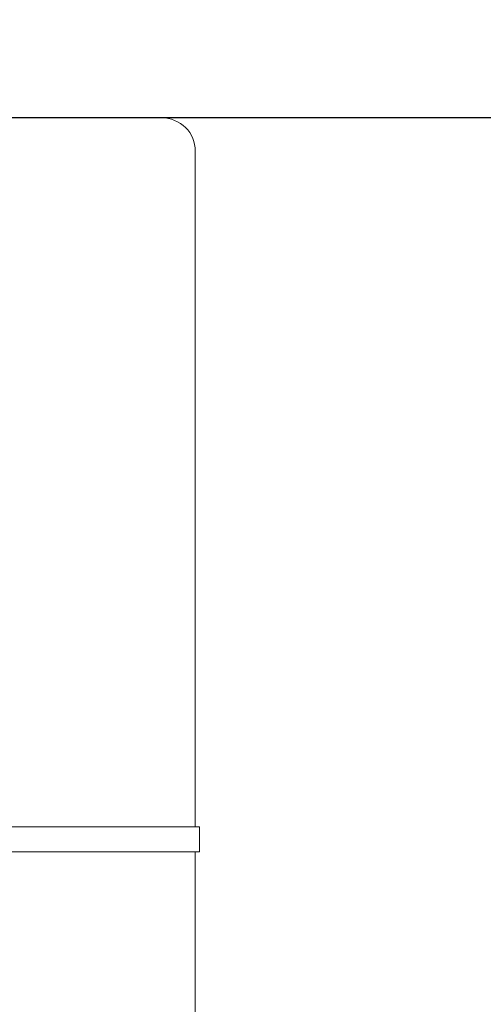
# Model space of a CAD drawing. Units: inches. Extents: x -1198 to -69, y -512 to 437.
# Tile 37 of 50: x -625.117 to -622.655, y 180.515 to 185.749. Entities that reach past the tile are written whole.
import ezdxf

# ---------------------------------------------------------------- set-up
doc = ezdxf.new("R2010")
doc.units = ezdxf.units.IN
doc.header["$MEASUREMENT"] = 0
for name, color, linetype, lineweight in [('0_Pen_No__7', 7, 'Continuous', 18), ('A-ANNO-DIMS', 2, 'Continuous', 18), ('A-EQPM', 60, 'Continuous', 18), ('A-FLOR-CASE', 7, 'Continuous', 25)]:
    doc.layers.add(name, color=color, linetype=linetype, lineweight=lineweight)
doc.styles.get("Standard").update_dxf_attribs({"font": 'arial.ttf'})
doc.dimstyles.get("Standard").update_dxf_attribs({"dimtxt": 6, "dimasz": 6, "dimexe": 0.18, "dimexo": 0.0625, "dimgap": 0.09, "dimtad": 0, "dimtih": 1, "dimtoh": 1, "dimdec": 0, "dimzin": 0, "dimdsep": 46, "dimlunit": 4, "dimtxsty": 'Standard', "dimblk": 'OBLIQUE', "dimcen": 0.09, "dimadec": 0, "dimazin": 0, "dimtfac": 1, "dimtdec": 0, "dimtofl": 0, "dimtmove": 0, "dimatfit": 3, "dimfxl": 1, "dimtolj": 1, "dimtzin": 0, "dimarcsym": 0})

# ---------------------------------------------------------------- blocks, each defined once
blk = doc.blocks.new('new block')
at = {"layer": '0_Pen_No__7'}
for p, q in [((-359, 99.11), (485.68, 99.11)), ((485.68, 95.73), (-359, 95.73))]:
    blk.add_line(p, q, dxfattribs=at)
blk.add_lwpolyline([(-354.49, 596.91), (481.18, 596.91, -0.414214), (485.68, 592.4), (485.68, 99.11), (486.24, 99.11), (486.24, 95.73), (485.68, 95.73), (485.68, 4.5, -0.414214), (481.18, 0), (-354.49, 0, -0.414214), (-359, 4.5), (-359, 95.73), (-359.56, 95.73), (-359.56, 99.11), (-359, 99.11), (-359, 592.4, -0.414214)], format="xyb", close=True, dxfattribs=at)
blk = doc.blocks.new('COUNTER-L')
at = {"ltscale": 10}
blk.add_line((49.3491, 23.9997), (0.0001, 23.9997), dxfattribs=at)
blk = doc.blocks.new('_Oblique')
at = {"color": 0, "linetype": 'ByBlock', "lineweight": -2}
blk.add_line((-0.5, -0.5), (0.5, 0.5), dxfattribs=at)
blk = doc.blocks.new('*D56')
at = {"layer": 'A-ANNO-DIMS', "color": 0, "lineweight": -2, "ltscale": 10, "transparency": 16777216}
for p, q in [((-618.3394, 257.2277), (-603.8219, 257.2277)), ((-604.0019, 257.2277), (-604.0019, 212.422)), ((-604.0019, 161.2277), (-604.0019, 206.0333)), ((-618.3394, 161.2277), (-603.8219, 161.2277))]:
    blk.add_line(p, q, dxfattribs=at)
at = {"layer": 'DEFPOINTS', "color": 0, "ltscale": 10, "transparency": 16777216}
for p in [(-618.4019, 257.2277), (-604.0019, 257.2277), (-618.4019, 161.2277)]:
    blk.add_point(p, dxfattribs=at)
at = {"layer": 'A-ANNO-DIMS', "color": 0, "lineweight": -2, "ltscale": 10, "transparency": 16777216, "xscale": 6, "yscale": 6, "zscale": 6}
for p, rotation in [((-604.0019, 257.2277), 90), ((-604.0019, 161.2277), 270)]:
    blk.add_blockref('_Oblique', p, dxfattribs=dict(at, rotation=rotation))
at = {"layer": 'A-ANNO-DIMS', "color": 0, "ltscale": 10, "transparency": 16777216, "insert": (-604.0019, 209.2277), "char_height": 6, "attachment_point": 5}
blk.add_mtext('\\A1;COUNTER 96 TYP.', dxfattribs=at)

msp = doc.modelspace()

# ---------------------------------------------------------------- block references
at = {"layer": 'A-EQPM', "xscale": 0.0393700787401575, "yscale": 0.0393700787401575, "zscale": 0.0393700787401575, "rotation": 180}
msp.add_blockref('new block', (-638.3186, 185.2277), dxfattribs=at)
at = {"layer": 'A-FLOR-CASE'}
msp.add_blockref('COUNTER-L', (-667.751, 161.228), dxfattribs=at)

# ---------------------------------------------------------------- dimensions: what is measured, and where the dimension line sits
at = {"layer": 'A-ANNO-DIMS', "ltscale": 10}
dim = msp.add_linear_dim(base=(-604.0019, 257.2277), p1=(-618.4019, 161.2277), p2=(-618.4019, 257.2277), angle=90, text='COUNTER <> TYP.', dimstyle='Standard', override={"dimdec": 0, "dimlfac": 1, "dimrnd": 0, "dimzin": 0, "dimdsep": 46, "dimlunit": 2}, dxfattribs=at)
dim.commit()
dim.dimension.update_dxf_attribs({"geometry": '*D56', "text_midpoint": (-604.0019, 209.2277)})

doc.saveas('drawing.dxf')
